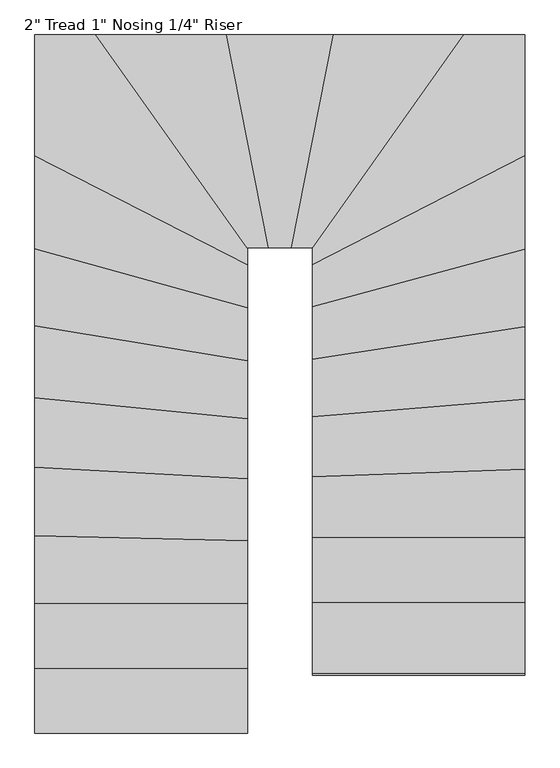
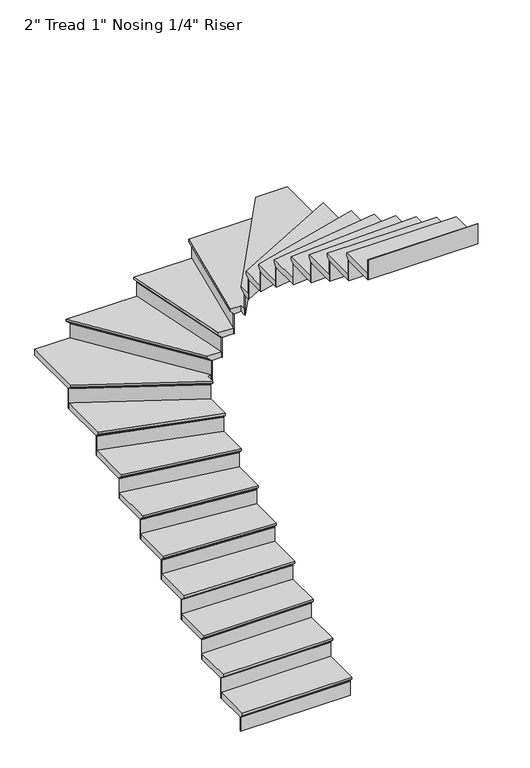
"""IFC4 building model written with IfcOpenShell, lengths in millimetres: stair flight geometry."""

from ifc_helpers import new_model, si_unit, origin, place, context, project, spatial, faceted_brep, source, transform, mapped, element, save


def stair_flight_cb62f9a1(model_context):
    return source(origin(), model_context, "Body", "Brep", [
        faceted_brep([(-7191.832922, 6052.3300735, 155.1214286), (-7191.832922, 6052.3300735, 174.1714286), (-8106.232922, 6052.3300735, 174.1714286), (-8106.232922, 6052.3300735, 155.1214286), (-7191.832922, 6077.7300735, 129.7214286), (-8106.232922, 6077.7300735, 129.7214286), (-7191.832922, 6357.1300735, 174.1714286), (-8106.232922, 6357.1300735, 174.1714286), (-8106.232922, 6077.7300735, 123.3714286), (-8106.232922, 6357.1300735, 123.3714286), (-7191.832922, 6357.1300735, 123.3714286), (-7191.832922, 6077.7300735, 123.3714286)], [[[0, 1, 2, 3]], [[4, 0, 3, 5]], [[2, 1, 6, 7]], [[8, 9, 10, 11]], [[2, 7, 9, 8, 5, 3]], [[8, 11, 4, 5]], [[6, 1, 0, 4, 11, 10]], [[7, 6, 10, 9]]]),
        faceted_brep([(-7191.832922, 6077.7300735, 123.3714286), (-7191.832922, 6077.7300735, 0.0), (-7191.832922, 6084.0800735, 0.0), (-7191.832922, 6084.0800735, 123.3714286), (-8106.232922, 6077.7300735, 123.3714286), (-8106.232922, 6084.0800735, 123.3714286), (-8106.232922, 6084.0800735, 0.0), (-8106.232922, 6077.7300735, 0.0)], [[[0, 1, 2, 3]], [[4, 5, 6, 7]], [[1, 0, 4, 7]], [[2, 1, 7, 6]], [[3, 2, 6, 5]], [[0, 3, 5, 4]]]),
        faceted_brep([(-7191.832922, 6357.1300735, 297.5428571), (-7191.832922, 6357.1300735, 123.3714286), (-7191.832922, 6363.4800735, 123.3714286), (-7191.832922, 6363.4800735, 297.5428571), (-8106.232922, 6357.1300735, 297.5428571), (-8106.232922, 6363.4800735, 297.5428571), (-8106.232922, 6363.4800735, 123.3714286), (-8106.232922, 6357.1300735, 123.3714286)], [[[0, 1, 2, 3]], [[4, 5, 6, 7]], [[1, 0, 4, 7]], [[2, 1, 7, 6]], [[3, 2, 6, 5]], [[0, 3, 5, 4]]]),
        faceted_brep([(-8106.232922, 6331.7300735, 348.3428571), (-7191.832922, 6331.7300735, 348.3428571), (-7191.832922, 6636.5300735, 348.3428571), (-8106.232922, 6636.5300735, 348.3428571), (-8106.232922, 6357.1300735, 297.5428571), (-8106.232922, 6636.5300735, 297.5428571), (-7191.832922, 6636.5300735, 297.5428571), (-7191.832922, 6357.1300735, 297.5428571), (-8106.232922, 6357.1300735, 303.8928571), (-8106.232922, 6331.7300735, 329.2928571), (-7191.832922, 6357.1300735, 303.8928571), (-7191.832922, 6331.7300735, 329.2928571)], [[[0, 1, 2, 3]], [[4, 5, 6, 7]], [[0, 3, 5, 4, 8, 9]], [[4, 7, 10, 8]], [[2, 1, 11, 10, 7, 6]], [[3, 2, 6, 5]], [[11, 1, 0, 9]], [[10, 11, 9, 8]]]),
        faceted_brep([(-7191.832922, 6636.5300735, 471.7142857), (-7191.832922, 6636.5300735, 297.5428571), (-7191.832922, 6642.8800735, 297.5428571), (-7191.832922, 6642.8800735, 471.7142857), (-8106.232922, 6636.5300735, 471.7142857), (-8106.232922, 6642.8800735, 471.7142857), (-8106.232922, 6642.8800735, 297.5428571), (-8106.232922, 6636.5300735, 297.5428571)], [[[0, 1, 2, 3]], [[4, 5, 6, 7]], [[1, 0, 4, 7]], [[2, 1, 7, 6]], [[3, 2, 6, 5]], [[0, 3, 5, 4]]]),
        faceted_brep([(-8106.232922, 6611.1300735, 522.5142857), (-7191.832922, 6611.1300735, 522.5142857), (-7191.832922, 6905.3290235, 522.5142857), (-8106.232922, 6926.5447952, 522.5142857), (-8106.232922, 6636.5300735, 471.7142857), (-8106.232922, 6926.5447952, 471.7142857), (-7191.832922, 6905.3290235, 471.7142857), (-7191.832922, 6636.5300735, 471.7142857), (-8106.232922, 6636.5300735, 478.0642857), (-8106.232922, 6611.1300735, 503.4642857), (-7191.832922, 6636.5300735, 478.0642857), (-7191.832922, 6611.1300735, 503.4642857)], [[[0, 1, 2, 3]], [[4, 5, 6, 7]], [[0, 3, 5, 4, 8, 9]], [[4, 7, 10, 8]], [[2, 1, 11, 10, 7, 6]], [[3, 2, 6, 5]], [[11, 1, 0, 9]], [[10, 11, 9, 8]]]),
        faceted_brep([(-7191.832922, 6905.3290235, 645.8857143), (-7191.832922, 6905.3290235, 471.7142857), (-7191.832922, 6911.6807324, 471.7142857), (-7191.832922, 6911.6807324, 645.8857143), (-8106.232922, 6926.5447952, 645.8857143), (-8106.232922, 6932.8965042, 645.8857143), (-8106.232922, 6932.8965042, 471.7142857), (-8106.232922, 6926.5447952, 471.7142857)], [[[0, 1, 2, 3]], [[4, 5, 6, 7]], [[1, 0, 4, 7]], [[2, 1, 7, 6]], [[3, 2, 6, 5]], [[0, 3, 5, 4]]]),
        faceted_brep([(-8106.232922, 6901.1379594, 696.6857143), (-7191.832922, 6879.9221876, 696.6857143), (-7191.832922, 7170.5442934, 696.6857143), (-8106.232922, 7220.1906734, 696.6857143), (-8106.232922, 6926.5447952, 645.8857143), (-8106.232922, 7220.1906734, 645.8857143), (-7191.832922, 7170.5442934, 645.8857143), (-7191.832922, 6905.3290235, 645.8857143), (-8106.232922, 6926.5447952, 652.2357143), (-8106.232922, 6901.1379594, 677.6357143), (-7191.832922, 6905.3290235, 652.2357143), (-7191.832922, 6879.9221876, 677.6357143)], [[[0, 1, 2, 3]], [[4, 5, 6, 7]], [[0, 3, 5, 4, 8, 9]], [[4, 7, 10, 8]], [[2, 1, 11, 10, 7, 6]], [[3, 2, 6, 5]], [[11, 1, 0, 9]], [[10, 11, 9, 8]]]),
        faceted_brep([(-7191.832922, 7170.5442934, 820.0571429), (-7191.832922, 7170.5442934, 645.8857143), (-7191.832922, 7176.9036459, 645.8857143), (-7191.832922, 7176.9036459, 820.0571429), (-8106.232922, 7220.1906734, 820.0571429), (-8106.232922, 7226.5500259, 820.0571429), (-8106.232922, 7226.5500259, 645.8857143), (-8106.232922, 7220.1906734, 645.8857143)], [[[0, 1, 2, 3]], [[4, 5, 6, 7]], [[1, 0, 4, 7]], [[2, 1, 7, 6]], [[3, 2, 6, 5]], [[0, 3, 5, 4]]]),
        faceted_brep([(-8106.232922, 7194.7532635, 870.8571429), (-7191.832922, 7145.1068835, 870.8571429), (-7191.832922, 7429.9889999, 870.8571429), (-8106.232922, 7519.7151289, 870.8571429), (-8106.232922, 7220.1906734, 820.0571429), (-8106.232922, 7519.7151289, 820.0571429), (-7191.832922, 7429.9889999, 820.0571429), (-7191.832922, 7170.5442934, 820.0571429), (-8106.232922, 7220.1906734, 826.4071429), (-8106.232922, 7194.7532635, 851.8071429), (-7191.832922, 7170.5442934, 826.4071429), (-7191.832922, 7145.1068835, 851.8071429)], [[[0, 1, 2, 3]], [[4, 5, 6, 7]], [[0, 3, 5, 4, 8, 9]], [[4, 7, 10, 8]], [[2, 1, 11, 10, 7, 6]], [[3, 2, 6, 5]], [[11, 1, 0, 9]], [[10, 11, 9, 8]]]),
        faceted_brep([(-7191.832922, 7429.9889999, 994.2285714), (-7191.832922, 7429.9889999, 820.0571429), (-7191.832922, 7436.3694976, 820.0571429), (-7191.832922, 7436.3694976, 994.2285714), (-8106.232922, 7519.7151289, 994.2285714), (-8106.232922, 7526.0956267, 994.2285714), (-8106.232922, 7526.0956267, 820.0571429), (-8106.232922, 7519.7151289, 820.0571429)], [[[0, 1, 2, 3]], [[4, 5, 6, 7]], [[1, 0, 4, 7]], [[2, 1, 7, 6]], [[3, 2, 6, 5]], [[0, 3, 5, 4]]]),
        faceted_brep([(-8106.232922, 7494.193138, 1045.0285714), (-7191.832922, 7404.467009, 1045.0285714), (-7191.832922, 7679.2419202, 1045.0285714), (-8106.232922, 7829.7013355, 1045.0285714), (-8106.232922, 7519.7151289, 994.2285714), (-8106.232922, 7829.7013355, 994.2285714), (-7191.832922, 7679.2419202, 994.2285714), (-7191.832922, 7429.9889999, 994.2285714), (-8106.232922, 7519.7151289, 1000.5785714), (-8106.232922, 7494.193138, 1025.9785714), (-7191.832922, 7429.9889999, 1000.5785714), (-7191.832922, 7404.467009, 1025.9785714)], [[[0, 1, 2, 3]], [[4, 5, 6, 7]], [[0, 3, 5, 4, 8, 9]], [[4, 7, 10, 8]], [[2, 1, 11, 10, 7, 6]], [[3, 2, 6, 5]], [[11, 1, 0, 9]], [[10, 11, 9, 8]]]),
        faceted_brep([(-7191.832922, 7679.2419202, 1168.4), (-7191.832922, 7679.2419202, 994.2285714), (-7191.832922, 7685.6773088, 994.2285714), (-7191.832922, 7685.6773088, 1168.4), (-8106.232922, 7829.7013355, 1168.4), (-8106.232922, 7836.1367241, 1168.4), (-8106.232922, 7836.1367241, 994.2285714), (-8106.232922, 7829.7013355, 994.2285714)], [[[0, 1, 2, 3]], [[4, 5, 6, 7]], [[1, 0, 4, 7]], [[2, 1, 7, 6]], [[3, 2, 6, 5]], [[0, 3, 5, 4]]]),
        faceted_brep([(-8106.232922, 7803.9597811, 1219.2), (-7191.832922, 7653.5003659, 1219.2), (-7191.832922, 7907.8111185, 1219.2), (-8106.232922, 8161.162863, 1219.2), (-8106.232922, 7829.7013355, 1168.4), (-8106.232922, 8161.162863, 1168.4), (-7191.832922, 7907.8111185, 1168.4), (-7191.832922, 7679.2419202, 1168.4), (-8106.232922, 7829.7013355, 1174.75), (-8106.232922, 7803.9597811, 1200.15), (-7191.832922, 7679.2419202, 1174.75), (-7191.832922, 7653.5003659, 1200.15)], [[[0, 1, 2, 3]], [[4, 5, 6, 7]], [[0, 3, 5, 4, 8, 9]], [[4, 7, 10, 8]], [[2, 1, 11, 10, 7, 6]], [[3, 2, 6, 5]], [[11, 1, 0, 9]], [[10, 11, 9, 8]]]),
        faceted_brep([(-7191.832922, 7907.8111185, 1342.5714286), (-7191.832922, 7907.8111185, 1168.4), (-7191.832922, 7914.4003479, 1168.4), (-7191.832922, 7914.4003479, 1342.5714286), (-8106.232922, 8161.162863, 1342.5714286), (-8106.232922, 8167.7520923, 1342.5714286), (-8106.232922, 8167.7520923, 1168.4), (-8106.232922, 8161.162863, 1168.4)], [[[0, 1, 2, 3]], [[4, 5, 6, 7]], [[1, 0, 4, 7]], [[2, 1, 7, 6]], [[3, 2, 6, 5]], [[0, 3, 5, 4]]]),
        faceted_brep([(-8106.232922, 8134.8059457, 1393.3714286), (-7191.832922, 7881.4542013, 1393.3714286), (-7191.832922, 8093.1377934, 1393.3714286), (-8106.232922, 8561.9624147, 1393.3714286), (-8106.232922, 8161.162863, 1342.5714286), (-8106.232922, 8561.9624147, 1342.5714286), (-7191.832922, 8093.1377934, 1342.5714286), (-7191.832922, 7907.8111185, 1342.5714286), (-8106.232922, 8161.162863, 1348.9214286), (-8106.232922, 8134.8059457, 1374.3214286), (-7191.832922, 7907.8111185, 1348.9214286), (-7191.832922, 7881.4542013, 1374.3214286)], [[[0, 1, 2, 3]], [[4, 5, 6, 7]], [[0, 3, 5, 4, 8, 9]], [[4, 7, 10, 8]], [[2, 1, 11, 10, 7, 6]], [[3, 2, 6, 5]], [[11, 1, 0, 9]], [[10, 11, 9, 8]]]),
        faceted_brep([(-7191.832922, 8093.1377934, 1516.7428571), (-7191.832922, 8093.1377934, 1342.5714286), (-7191.832922, 8100.2737765, 1342.5714286), (-7191.832922, 8100.2737765, 1516.7428571), (-8106.232922, 8561.9624147, 1516.7428571), (-8106.232922, 8569.0983978, 1516.7428571), (-8106.232922, 8569.0983978, 1342.5714286), (-8106.232922, 8561.9624147, 1342.5714286)], [[[0, 1, 2, 3]], [[4, 5, 6, 7]], [[1, 0, 4, 7]], [[2, 1, 7, 6]], [[3, 2, 6, 5]], [[0, 3, 5, 4]]]),
        faceted_brep([(-7812.5517883, 9053.2617654, 1567.5428571), (-8106.232922, 9053.2617654, 1567.5428571), (-8106.232922, 8533.4184821, 1567.5428571), (-7191.832922, 8064.5938608, 1567.5428571), (-7191.832922, 8138.8617654, 1567.5428571), (-7162.2778392, 8138.8617654, 1567.5428571), (-8106.232922, 9053.2617654, 1516.7428571), (-7812.5517883, 9053.2617654, 1516.7428571), (-7162.2778392, 8138.8617654, 1516.7428571), (-7191.832922, 8138.8617654, 1516.7428571), (-7191.832922, 8093.1377934, 1516.7428571), (-8106.232922, 8561.9624147, 1516.7428571), (-8106.232922, 8561.9624147, 1523.0928571), (-8106.232922, 8533.4184821, 1548.4928571), (-7191.832922, 8093.1377934, 1523.0928571), (-7191.832922, 8064.5938608, 1548.4928571)], [[[0, 1, 2, 3, 4, 5]], [[6, 7, 8, 9, 10, 11]], [[1, 0, 7, 6]], [[2, 1, 6, 11, 12, 13]], [[11, 10, 14, 12]], [[4, 3, 15, 14, 10, 9]], [[5, 4, 9, 8]], [[0, 5, 8, 7]], [[15, 3, 2, 13]], [[14, 15, 13, 12]]]),
        faceted_brep([(-7162.2778392, 8138.8617654, 1690.9142857), (-7162.2778392, 8138.8617654, 1516.7428571), (-7154.4858644, 8138.8617654, 1516.7428571), (-7154.4858644, 8138.8617654, 1690.9142857), (-7812.5517883, 9053.2617654, 1690.9142857), (-7804.7598135, 9053.2617654, 1690.9142857), (-7804.7598135, 9053.2617654, 1516.7428571), (-7812.5517883, 9053.2617654, 1516.7428571)], [[[0, 1, 2, 3]], [[4, 5, 6, 7]], [[1, 0, 4, 7]], [[2, 1, 7, 6]], [[3, 2, 6, 5]], [[0, 3, 5, 4]]]),
        faceted_brep([(-7843.7196875, 9053.2617654, 1741.7142857), (-7193.4457383, 8138.8617654, 1741.7142857), (-7075.8237521, 8138.8617654, 1741.7142857), (-7256.0646084, 9053.2617654, 1741.7142857), (-7812.5517883, 9053.2617654, 1690.9142857), (-7256.0646084, 9053.2617654, 1690.9142857), (-7075.8237521, 8138.8617654, 1690.9142857), (-7162.2778392, 8138.8617654, 1690.9142857), (-7812.5517883, 9053.2617654, 1697.2642857), (-7843.7196875, 9053.2617654, 1722.6642857), (-7162.2778392, 8138.8617654, 1697.2642857), (-7193.4457383, 8138.8617654, 1722.6642857)], [[[0, 1, 2, 3]], [[4, 5, 6, 7]], [[0, 3, 5, 4, 8, 9]], [[4, 7, 10, 8]], [[2, 1, 11, 10, 7, 6]], [[3, 2, 6, 5]], [[11, 1, 0, 9]], [[10, 11, 9, 8]]]),
        faceted_brep([(-7075.8237521, 8138.8617654, 1865.0857143), (-7075.8237521, 8138.8617654, 1690.9142857), (-7069.3515667, 8138.8617654, 1690.9142857), (-7069.3515667, 8138.8617654, 1865.0857143), (-7256.0646084, 9053.2617654, 1865.0857143), (-7249.592423, 9053.2617654, 1865.0857143), (-7249.592423, 9053.2617654, 1690.9142857), (-7256.0646084, 9053.2617654, 1690.9142857)], [[[0, 1, 2, 3]], [[4, 5, 6, 7]], [[1, 0, 4, 7]], [[2, 1, 7, 6]], [[3, 2, 6, 5]], [[0, 3, 5, 4]]]),
        faceted_brep([(-7281.9533502, 9053.2617654, 1915.8857143), (-7101.7124938, 8138.8617654, 1915.8857143), (-6976.6646084, 8138.8617654, 1915.8857143), (-6796.4237521, 9053.2617654, 1915.8857143), (-7256.0646084, 9053.2617654, 1865.0857143), (-6796.4237521, 9053.2617654, 1865.0857143), (-6976.6646084, 8138.8617654, 1865.0857143), (-7075.8237521, 8138.8617654, 1865.0857143), (-7256.0646084, 9053.2617654, 1871.4357143), (-7281.9533502, 9053.2617654, 1896.8357143), (-7075.8237521, 8138.8617654, 1871.4357143), (-7101.7124938, 8138.8617654, 1896.8357143)], [[[0, 1, 2, 3]], [[4, 5, 6, 7]], [[0, 3, 5, 4, 8, 9]], [[4, 7, 10, 8]], [[2, 1, 11, 10, 7, 6]], [[3, 2, 6, 5]], [[11, 1, 0, 9]], [[10, 11, 9, 8]]]),
        faceted_brep([(-6976.6646084, 8138.8617654, 2039.2571429), (-6976.6646084, 8138.8617654, 1865.0857143), (-6970.192423, 8138.8617654, 1865.0857143), (-6970.192423, 8138.8617654, 2039.2571429), (-6796.4237521, 9053.2617654, 2039.2571429), (-6789.9515667, 9053.2617654, 2039.2571429), (-6789.9515667, 9053.2617654, 1865.0857143), (-6796.4237521, 9053.2617654, 1865.0857143)], [[[0, 1, 2, 3]], [[4, 5, 6, 7]], [[1, 0, 4, 7]], [[2, 1, 7, 6]], [[3, 2, 6, 5]], [[0, 3, 5, 4]]]),
        faceted_brep([(-6822.3124938, 9053.2617654, 2090.0571429), (-7002.5533502, 8138.8617654, 2090.0571429), (-6912.432922, 8138.8617654, 2090.0571429), (-6912.432922, 8092.7662908, 2090.0571429), (-6229.3782573, 9053.2617654, 2090.0571429), (-6796.4237521, 9053.2617654, 2039.2571429), (-6229.3782573, 9053.2617654, 2039.2571429), (-6912.432922, 8092.7662908, 2039.2571429), (-6912.432922, 8138.8617654, 2039.2571429), (-6976.6646084, 8138.8617654, 2039.2571429), (-6796.4237521, 9053.2617654, 2045.6071429), (-6822.3124938, 9053.2617654, 2071.0071429), (-6976.6646084, 8138.8617654, 2045.6071429), (-7002.5533502, 8138.8617654, 2071.0071429)], [[[0, 1, 2, 3, 4]], [[5, 6, 7, 8, 9]], [[0, 4, 6, 5, 10, 11]], [[5, 9, 12, 10]], [[2, 1, 13, 12, 9, 8]], [[3, 2, 8, 7]], [[4, 3, 7, 6]], [[13, 1, 0, 11]], [[12, 13, 11, 10]]]),
        faceted_brep([(-6912.432922, 8092.7662908, 2213.4285714), (-6912.432922, 8092.7662908, 2039.2571429), (-6912.432922, 8081.8093984, 2039.2571429), (-6912.432922, 8081.8093984, 2213.4285714), (-6229.3782573, 9053.2617654, 2213.4285714), (-6221.5862826, 9053.2617654, 2213.4285714), (-6221.5862826, 9053.2617654, 2039.2571429), (-6229.3782573, 9053.2617654, 2039.2571429)], [[[0, 1, 2, 3]], [[4, 5, 6, 7]], [[1, 0, 4, 7]], [[2, 1, 7, 6]], [[3, 2, 6, 5]], [[0, 3, 5, 4]]]),
        faceted_brep([(-5998.032922, 8504.8745496, 2264.2285714), (-5998.032922, 9053.2617654, 2264.2285714), (-6260.5461565, 9053.2617654, 2264.2285714), (-6912.432922, 8136.5938608, 2264.2285714), (-6912.432922, 8036.0499283, 2264.2285714), (-5998.032922, 9053.2617654, 2213.4285714), (-5998.032922, 8504.8745496, 2213.4285714), (-6912.432922, 8036.0499283, 2213.4285714), (-6912.432922, 8092.7662908, 2213.4285714), (-6229.3782573, 9053.2617654, 2213.4285714), (-6229.3782573, 9053.2617654, 2219.7785714), (-6260.5461565, 9053.2617654, 2245.1785714), (-6912.432922, 8092.7662908, 2219.7785714), (-6912.432922, 8136.5938608, 2245.1785714)], [[[0, 1, 2, 3, 4]], [[5, 6, 7, 8, 9]], [[1, 0, 6, 5]], [[2, 1, 5, 9, 10, 11]], [[9, 8, 12, 10]], [[4, 3, 13, 12, 8, 7]], [[0, 4, 7, 6]], [[13, 3, 2, 11]], [[12, 13, 11, 10]]]),
        faceted_brep([(-6912.432922, 8036.0499283, 2387.6), (-6912.432922, 8036.0499283, 2213.4285714), (-6912.432922, 8028.9139451, 2213.4285714), (-6912.432922, 8028.9139451, 2387.6), (-5998.032922, 8504.8745496, 2387.6), (-5998.032922, 8497.7385665, 2387.6), (-5998.032922, 8497.7385665, 2213.4285714), (-5998.032922, 8504.8745496, 2213.4285714)], [[[0, 1, 2, 3]], [[4, 5, 6, 7]], [[1, 0, 4, 7]], [[2, 1, 7, 6]], [[3, 2, 6, 5]], [[0, 3, 5, 4]]]),
        faceted_brep([(-5998.032922, 8533.4184821, 2438.4), (-6912.432922, 8064.5938608, 2438.4), (-6912.432922, 7858.7269466, 2438.4), (-5998.032922, 8104.9241016, 2438.4), (-5998.032922, 8504.8745496, 2387.6), (-5998.032922, 8104.9241016, 2387.6), (-6912.432922, 7858.7269466, 2387.6), (-6912.432922, 8036.0499283, 2387.6), (-5998.032922, 8504.8745496, 2393.95), (-5998.032922, 8533.4184821, 2419.35), (-6912.432922, 8036.0499283, 2393.95), (-6912.432922, 8064.5938608, 2419.35)], [[[0, 1, 2, 3]], [[4, 5, 6, 7]], [[0, 3, 5, 4, 8, 9]], [[4, 7, 10, 8]], [[2, 1, 11, 10, 7, 6]], [[3, 2, 6, 5]], [[11, 1, 0, 9]], [[10, 11, 9, 8]]]),
        faceted_brep([(-6912.432922, 7858.7269466, 2561.7714286), (-6912.432922, 7858.7269466, 2387.6), (-6912.432922, 7852.1508092, 2387.6), (-6912.432922, 7852.1508092, 2561.7714286), (-5998.032922, 8104.9241016, 2561.7714286), (-5998.032922, 8098.3479643, 2561.7714286), (-5998.032922, 8098.3479643, 2387.6), (-5998.032922, 8104.9241016, 2387.6)], [[[0, 1, 2, 3]], [[4, 5, 6, 7]], [[1, 0, 4, 7]], [[2, 1, 7, 6]], [[3, 2, 6, 5]], [[0, 3, 5, 4]]]),
        faceted_brep([(-5998.032922, 8131.228651, 2612.5714286), (-6912.432922, 7885.031496, 2612.5714286), (-6912.432922, 7634.0506742, 2612.5714286), (-5998.032922, 7772.034344, 2612.5714286), (-5998.032922, 8104.9241016, 2561.7714286), (-5998.032922, 7772.034344, 2561.7714286), (-6912.432922, 7634.0506742, 2561.7714286), (-6912.432922, 7858.7269466, 2561.7714286), (-5998.032922, 8104.9241016, 2568.1214286), (-5998.032922, 8131.228651, 2593.5214286), (-6912.432922, 7858.7269466, 2568.1214286), (-6912.432922, 7885.031496, 2593.5214286)], [[[0, 1, 2, 3]], [[4, 5, 6, 7]], [[0, 3, 5, 4, 8, 9]], [[4, 7, 10, 8]], [[2, 1, 11, 10, 7, 6]], [[3, 2, 6, 5]], [[11, 1, 0, 9]], [[10, 11, 9, 8]]]),
        faceted_brep([(-6912.432922, 7634.0506742, 2735.9428571), (-6912.432922, 7634.0506742, 2561.7714286), (-6912.432922, 7627.6287831, 2561.7714286), (-6912.432922, 7627.6287831, 2735.9428571), (-5998.032922, 7772.034344, 2735.9428571), (-5998.032922, 7765.6124529, 2735.9428571), (-5998.032922, 7765.6124529, 2561.7714286), (-5998.032922, 7772.034344, 2561.7714286)], [[[0, 1, 2, 3]], [[4, 5, 6, 7]], [[1, 0, 4, 7]], [[2, 1, 7, 6]], [[3, 2, 6, 5]], [[0, 3, 5, 4]]]),
        faceted_brep([(-5998.032922, 7797.7219084, 2786.7428571), (-6912.432922, 7659.7382386, 2786.7428571), (-6912.432922, 7387.1325491, 2786.7428571), (-5998.032922, 7460.5640566, 2786.7428571), (-5998.032922, 7772.034344, 2735.9428571), (-5998.032922, 7460.5640566, 2735.9428571), (-6912.432922, 7387.1325491, 2735.9428571), (-6912.432922, 7634.0506742, 2735.9428571), (-5998.032922, 7772.034344, 2742.2928571), (-5998.032922, 7797.7219084, 2767.6928571), (-6912.432922, 7634.0506742, 2742.2928571), (-6912.432922, 7659.7382386, 2767.6928571)], [[[0, 1, 2, 3]], [[4, 5, 6, 7]], [[0, 3, 5, 4, 8, 9]], [[4, 7, 10, 8]], [[2, 1, 11, 10, 7, 6]], [[3, 2, 6, 5]], [[11, 1, 0, 9]], [[10, 11, 9, 8]]]),
        faceted_brep([(-6912.432922, 7387.1325491, 2910.1142857), (-6912.432922, 7387.1325491, 2735.9428571), (-6912.432922, 7380.7621064, 2735.9428571), (-6912.432922, 7380.7621064, 2910.1142857), (-5998.032922, 7460.5640566, 2910.1142857), (-5998.032922, 7454.1936139, 2910.1142857), (-5998.032922, 7454.1936139, 2735.9428571), (-5998.032922, 7460.5640566, 2735.9428571)], [[[0, 1, 2, 3]], [[4, 5, 6, 7]], [[1, 0, 4, 7]], [[2, 1, 7, 6]], [[3, 2, 6, 5]], [[0, 3, 5, 4]]]),
        faceted_brep([(-5998.032922, 7486.0458273, 2960.9142857), (-6912.432922, 7412.6143198, 2960.9142857), (-6912.432922, 7129.2397806, 2960.9142857), (-5998.032922, 7159.7920182, 2960.9142857), (-5998.032922, 7460.5640566, 2910.1142857), (-5998.032922, 7159.7920182, 2910.1142857), (-6912.432922, 7129.2397806, 2910.1142857), (-6912.432922, 7387.1325491, 2910.1142857), (-5998.032922, 7460.5640566, 2916.4642857), (-5998.032922, 7486.0458273, 2941.8642857), (-6912.432922, 7387.1325491, 2916.4642857), (-6912.432922, 7412.6143198, 2941.8642857)], [[[0, 1, 2, 3]], [[4, 5, 6, 7]], [[0, 3, 5, 4, 8, 9]], [[4, 7, 10, 8]], [[2, 1, 11, 10, 7, 6]], [[3, 2, 6, 5]], [[11, 1, 0, 9]], [[10, 11, 9, 8]]]),
        faceted_brep([(-6912.432922, 7129.2397806, 3084.2857143), (-6912.432922, 7129.2397806, 2910.1142857), (-6912.432922, 7122.886237, 2910.1142857), (-6912.432922, 7122.886237, 3084.2857143), (-5998.032922, 7159.7920182, 3084.2857143), (-5998.032922, 7153.4384747, 3084.2857143), (-5998.032922, 7153.4384747, 2910.1142857), (-5998.032922, 7159.7920182, 2910.1142857)], [[[0, 1, 2, 3]], [[4, 5, 6, 7]], [[1, 0, 4, 7]], [[2, 1, 7, 6]], [[3, 2, 6, 5]], [[0, 3, 5, 4]]]),
        faceted_brep([(-5998.032922, 7185.2061923, 3135.0857143), (-6912.432922, 7154.6539547, 3135.0857143), (-6912.432922, 6865.1300735, 3135.0857143), (-5998.032922, 6865.1300735, 3135.0857143), (-5998.032922, 7159.7920182, 3084.2857143), (-5998.032922, 6865.1300735, 3084.2857143), (-6912.432922, 6865.1300735, 3084.2857143), (-6912.432922, 7129.2397806, 3084.2857143), (-5998.032922, 7159.7920182, 3090.6357143), (-5998.032922, 7185.2061923, 3116.0357143), (-6912.432922, 7129.2397806, 3090.6357143), (-6912.432922, 7154.6539547, 3116.0357143)], [[[0, 1, 2, 3]], [[4, 5, 6, 7]], [[0, 3, 5, 4, 8, 9]], [[4, 7, 10, 8]], [[2, 1, 11, 10, 7, 6]], [[3, 2, 6, 5]], [[11, 1, 0, 9]], [[10, 11, 9, 8]]]),
        faceted_brep([(-6912.432922, 6865.1300735, 3258.4571429), (-6912.432922, 6865.1300735, 3084.2857143), (-6912.432922, 6858.7800735, 3084.2857143), (-6912.432922, 6858.7800735, 3258.4571429), (-5998.032922, 6865.1300735, 3258.4571429), (-5998.032922, 6858.7800735, 3258.4571429), (-5998.032922, 6858.7800735, 3084.2857143), (-5998.032922, 6865.1300735, 3084.2857143)], [[[0, 1, 2, 3]], [[4, 5, 6, 7]], [[1, 0, 4, 7]], [[2, 1, 7, 6]], [[3, 2, 6, 5]], [[0, 3, 5, 4]]]),
        faceted_brep([(-5998.032922, 6890.5300735, 3309.2571429), (-6912.432922, 6890.5300735, 3309.2571429), (-6912.432922, 6585.7300735, 3309.2571429), (-5998.032922, 6585.7300735, 3309.2571429), (-5998.032922, 6865.1300735, 3258.4571429), (-5998.032922, 6585.7300735, 3258.4571429), (-6912.432922, 6585.7300735, 3258.4571429), (-6912.432922, 6865.1300735, 3258.4571429), (-5998.032922, 6865.1300735, 3264.8071429), (-5998.032922, 6890.5300735, 3290.2071429), (-6912.432922, 6865.1300735, 3264.8071429), (-6912.432922, 6890.5300735, 3290.2071429)], [[[0, 1, 2, 3]], [[4, 5, 6, 7]], [[0, 3, 5, 4, 8, 9]], [[4, 7, 10, 8]], [[2, 1, 11, 10, 7, 6]], [[3, 2, 6, 5]], [[11, 1, 0, 9]], [[10, 11, 9, 8]]]),
        faceted_brep([(-6912.432922, 6585.7300735, 3432.6285714), (-6912.432922, 6585.7300735, 3258.4571429), (-6912.432922, 6579.3800735, 3258.4571429), (-6912.432922, 6579.3800735, 3432.6285714), (-5998.032922, 6585.7300735, 3432.6285714), (-5998.032922, 6579.3800735, 3432.6285714), (-5998.032922, 6579.3800735, 3258.4571429), (-5998.032922, 6585.7300735, 3258.4571429)], [[[0, 1, 2, 3]], [[4, 5, 6, 7]], [[1, 0, 4, 7]], [[2, 1, 7, 6]], [[3, 2, 6, 5]], [[0, 3, 5, 4]]]),
        faceted_brep([(-6912.432922, 6306.3300735, 3606.8), (-6912.432922, 6306.3300735, 3432.6285714), (-6912.432922, 6299.9800735, 3432.6285714), (-6912.432922, 6299.9800735, 3606.8), (-5998.032922, 6306.3300735, 3606.8), (-5998.032922, 6299.9800735, 3606.8), (-5998.032922, 6299.9800735, 3432.6285714), (-5998.032922, 6306.3300735, 3432.6285714)], [[[0, 1, 2, 3]], [[4, 5, 6, 7]], [[1, 0, 4, 7]], [[2, 1, 7, 6]], [[3, 2, 6, 5]], [[0, 3, 5, 4]]]),
        faceted_brep([(-5998.032922, 6611.1300735, 3483.4285714), (-6912.432922, 6611.1300735, 3483.4285714), (-6912.432922, 6306.3300735, 3483.4285714), (-5998.032922, 6306.3300735, 3483.4285714), (-5998.032922, 6585.7300735, 3432.6285714), (-5998.032922, 6306.3300735, 3432.6285714), (-6912.432922, 6306.3300735, 3432.6285714), (-6912.432922, 6585.7300735, 3432.6285714), (-5998.032922, 6585.7300735, 3438.9785714), (-5998.032922, 6611.1300735, 3464.3785714), (-6912.432922, 6585.7300735, 3438.9785714), (-6912.432922, 6611.1300735, 3464.3785714)], [[[0, 1, 2, 3]], [[4, 5, 6, 7]], [[0, 3, 5, 4, 8, 9]], [[4, 7, 10, 8]], [[2, 1, 11, 10, 7, 6]], [[3, 2, 6, 5]], [[11, 1, 0, 9]], [[10, 11, 9, 8]]]),
    ])


if __name__ == "__main__":
    model = new_model("IFC4")
    model_context = context("Model", 3, world=origin())
    ifc_project = project(units=[si_unit("LENGTHUNIT", "METRE", prefix="MILLI")], contexts=[model_context])
    site = spatial("IfcSite", under=ifc_project)
    building = spatial("IfcBuilding", under=site)
    placement = place(None, origin())
    stair_flight_shape = stair_flight_cb62f9a1(model_context)
    element("IfcStairFlight", 1, ObjectType="2\" Tread 1\" Nosing 1/4\" Riser", at=placement, inside=building, context=model_context, shape_type="MappedRepresentation", body=[
        mapped(stair_flight_shape, transform((0.0, 0.0, 0.0), x_axis=(1.0, 0.0, 0.0), y_axis=(0.0, 1.0, 0.0), z_axis=(0.0, 0.0, 1.0))),
    ])
    save(model, "model.ifc")
